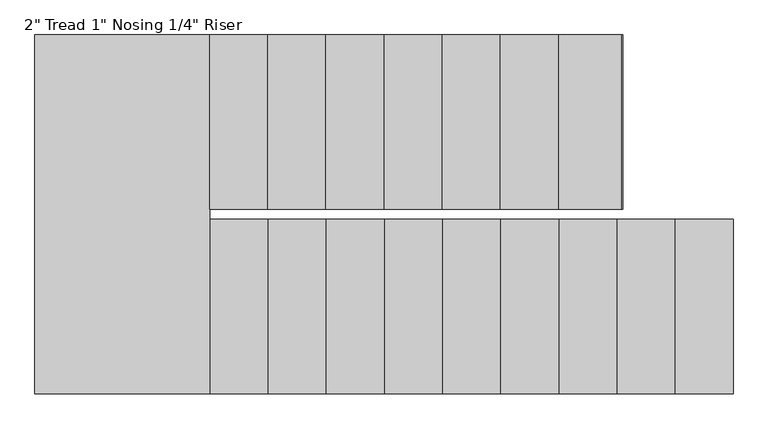
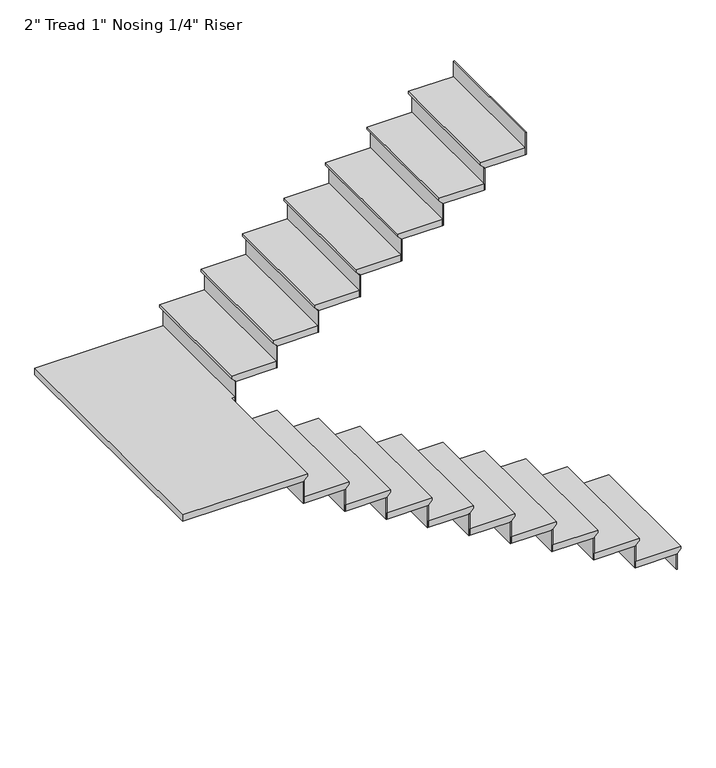
"""IFC4 building model written with IfcOpenShell, lengths in millimetres: stair flight geometry."""

from ifc_helpers import new_model, si_unit, origin, place, context, project, spatial, faceted_brep, source, transform, mapped, element, save


def stair_flight_03b7873a(model_context):
    return source(origin(), model_context, "Body", "Brep", [
        faceted_brep([(-5811.9482439, 2811.8172538, 3503.0833333), (-5811.9482439, 2811.8172538, 3522.1333333), (-5811.9482439, 1897.4172538, 3522.1333333), (-5811.9482439, 1897.4172538, 3503.0833333), (-5837.3482439, 2811.8172538, 3477.6833333), (-5837.3482439, 1897.4172538, 3477.6833333), (-6142.1482439, 2811.8172538, 3522.1333333), (-6142.1482439, 1897.4172538, 3522.1333333), (-5837.3482439, 1897.4172538, 3471.3333333), (-6142.1482439, 1897.4172538, 3471.3333333), (-6142.1482439, 2811.8172538, 3471.3333333), (-5837.3482439, 2811.8172538, 3471.3333333)], [[[0, 1, 2, 3]], [[4, 0, 3, 5]], [[2, 1, 6, 7]], [[8, 9, 10, 11]], [[2, 7, 9, 8, 5, 3]], [[8, 11, 4, 5]], [[6, 1, 0, 4, 11, 10]], [[7, 6, 10, 9]]]),
        faceted_brep([(-5837.3482439, 2811.8172538, 3471.3333333), (-5837.3482439, 2811.8172538, 3352.8), (-5843.6982439, 2811.8172538, 3352.8), (-5843.6982439, 2811.8172538, 3471.3333333), (-5837.3482439, 1897.4172538, 3471.3333333), (-5843.6982439, 1897.4172538, 3471.3333333), (-5843.6982439, 1897.4172538, 3352.8), (-5837.3482439, 1897.4172538, 3352.8)], [[[0, 1, 2, 3]], [[4, 5, 6, 7]], [[1, 0, 4, 7]], [[2, 1, 7, 6]], [[3, 2, 6, 5]], [[0, 3, 5, 4]]]),
        faceted_brep([(-6142.1482439, 2811.8172538, 3640.6666667), (-6142.1482439, 2811.8172538, 3471.3333333), (-6148.4982439, 2811.8172538, 3471.3333333), (-6148.4982439, 2811.8172538, 3640.6666667), (-6142.1482439, 1897.4172538, 3640.6666667), (-6148.4982439, 1897.4172538, 3640.6666667), (-6148.4982439, 1897.4172538, 3471.3333333), (-6142.1482439, 1897.4172538, 3471.3333333)], [[[0, 1, 2, 3]], [[4, 5, 6, 7]], [[1, 0, 4, 7]], [[2, 1, 7, 6]], [[3, 2, 6, 5]], [[0, 3, 5, 4]]]),
        faceted_brep([(-6116.7482439, 1897.4172538, 3691.4666667), (-6116.7482439, 2811.8172538, 3691.4666667), (-6446.9482439, 2811.8172538, 3691.4666667), (-6446.9482439, 1897.4172538, 3691.4666667), (-6142.1482439, 1897.4172538, 3640.6666667), (-6446.9482439, 1897.4172538, 3640.6666667), (-6446.9482439, 2811.8172538, 3640.6666667), (-6142.1482439, 2811.8172538, 3640.6666667), (-6142.1482439, 1897.4172538, 3647.0166667), (-6116.7482439, 1897.4172538, 3672.4166667), (-6142.1482439, 2811.8172538, 3647.0166667), (-6116.7482439, 2811.8172538, 3672.4166667)], [[[0, 1, 2, 3]], [[4, 5, 6, 7]], [[0, 3, 5, 4, 8, 9]], [[4, 7, 10, 8]], [[2, 1, 11, 10, 7, 6]], [[3, 2, 6, 5]], [[11, 1, 0, 9]], [[10, 11, 9, 8]]]),
        faceted_brep([(-6446.9482439, 2811.8172538, 3810.0), (-6446.9482439, 2811.8172538, 3640.6666667), (-6453.2982439, 2811.8172538, 3640.6666667), (-6453.2982439, 2811.8172538, 3810.0), (-6446.9482439, 1897.4172538, 3810.0), (-6453.2982439, 1897.4172538, 3810.0), (-6453.2982439, 1897.4172538, 3640.6666667), (-6446.9482439, 1897.4172538, 3640.6666667)], [[[0, 1, 2, 3]], [[4, 5, 6, 7]], [[1, 0, 4, 7]], [[2, 1, 7, 6]], [[3, 2, 6, 5]], [[0, 3, 5, 4]]]),
        faceted_brep([(-6421.5482439, 1897.4172538, 3860.8), (-6421.5482439, 2811.8172538, 3860.8), (-6751.7482439, 2811.8172538, 3860.8), (-6751.7482439, 1897.4172538, 3860.8), (-6446.9482439, 1897.4172538, 3810.0), (-6751.7482439, 1897.4172538, 3810.0), (-6751.7482439, 2811.8172538, 3810.0), (-6446.9482439, 2811.8172538, 3810.0), (-6446.9482439, 1897.4172538, 3816.35), (-6421.5482439, 1897.4172538, 3841.75), (-6446.9482439, 2811.8172538, 3816.35), (-6421.5482439, 2811.8172538, 3841.75)], [[[0, 1, 2, 3]], [[4, 5, 6, 7]], [[0, 3, 5, 4, 8, 9]], [[4, 7, 10, 8]], [[2, 1, 11, 10, 7, 6]], [[3, 2, 6, 5]], [[11, 1, 0, 9]], [[10, 11, 9, 8]]]),
        faceted_brep([(-6751.7482439, 2811.8172538, 3979.3333333), (-6751.7482439, 2811.8172538, 3810.0), (-6758.0982439, 2811.8172538, 3810.0), (-6758.0982439, 2811.8172538, 3979.3333333), (-6751.7482439, 1897.4172538, 3979.3333333), (-6758.0982439, 1897.4172538, 3979.3333333), (-6758.0982439, 1897.4172538, 3810.0), (-6751.7482439, 1897.4172538, 3810.0)], [[[0, 1, 2, 3]], [[4, 5, 6, 7]], [[1, 0, 4, 7]], [[2, 1, 7, 6]], [[3, 2, 6, 5]], [[0, 3, 5, 4]]]),
        faceted_brep([(-6726.3482439, 1897.4172538, 4030.1333333), (-6726.3482439, 2811.8172538, 4030.1333333), (-7056.5482439, 2811.8172538, 4030.1333333), (-7056.5482439, 1897.4172538, 4030.1333333), (-6751.7482439, 1897.4172538, 3979.3333333), (-7056.5482439, 1897.4172538, 3979.3333333), (-7056.5482439, 2811.8172538, 3979.3333333), (-6751.7482439, 2811.8172538, 3979.3333333), (-6751.7482439, 1897.4172538, 3985.6833333), (-6726.3482439, 1897.4172538, 4011.0833333), (-6751.7482439, 2811.8172538, 3985.6833333), (-6726.3482439, 2811.8172538, 4011.0833333)], [[[0, 1, 2, 3]], [[4, 5, 6, 7]], [[0, 3, 5, 4, 8, 9]], [[4, 7, 10, 8]], [[2, 1, 11, 10, 7, 6]], [[3, 2, 6, 5]], [[11, 1, 0, 9]], [[10, 11, 9, 8]]]),
        faceted_brep([(-7056.5482439, 2811.8172538, 4148.6666667), (-7056.5482439, 2811.8172538, 3979.3333333), (-7062.8982439, 2811.8172538, 3979.3333333), (-7062.8982439, 2811.8172538, 4148.6666667), (-7056.5482439, 1897.4172538, 4148.6666667), (-7062.8982439, 1897.4172538, 4148.6666667), (-7062.8982439, 1897.4172538, 3979.3333333), (-7056.5482439, 1897.4172538, 3979.3333333)], [[[0, 1, 2, 3]], [[4, 5, 6, 7]], [[1, 0, 4, 7]], [[2, 1, 7, 6]], [[3, 2, 6, 5]], [[0, 3, 5, 4]]]),
        faceted_brep([(-7031.1482439, 1897.4172538, 4199.4666667), (-7031.1482439, 2811.8172538, 4199.4666667), (-7361.3482439, 2811.8172538, 4199.4666667), (-7361.3482439, 1897.4172538, 4199.4666667), (-7056.5482439, 1897.4172538, 4148.6666667), (-7361.3482439, 1897.4172538, 4148.6666667), (-7361.3482439, 2811.8172538, 4148.6666667), (-7056.5482439, 2811.8172538, 4148.6666667), (-7056.5482439, 1897.4172538, 4155.0166667), (-7031.1482439, 1897.4172538, 4180.4166667), (-7056.5482439, 2811.8172538, 4155.0166667), (-7031.1482439, 2811.8172538, 4180.4166667)], [[[0, 1, 2, 3]], [[4, 5, 6, 7]], [[0, 3, 5, 4, 8, 9]], [[4, 7, 10, 8]], [[2, 1, 11, 10, 7, 6]], [[3, 2, 6, 5]], [[11, 1, 0, 9]], [[10, 11, 9, 8]]]),
        faceted_brep([(-7361.3482439, 2811.8172538, 4318.0), (-7361.3482439, 2811.8172538, 4148.6666667), (-7367.6982439, 2811.8172538, 4148.6666667), (-7367.6982439, 2811.8172538, 4318.0), (-7361.3482439, 1897.4172538, 4318.0), (-7367.6982439, 1897.4172538, 4318.0), (-7367.6982439, 1897.4172538, 4148.6666667), (-7361.3482439, 1897.4172538, 4148.6666667)], [[[0, 1, 2, 3]], [[4, 5, 6, 7]], [[1, 0, 4, 7]], [[2, 1, 7, 6]], [[3, 2, 6, 5]], [[0, 3, 5, 4]]]),
        faceted_brep([(-7335.9482439, 1897.4172538, 4368.8), (-7335.9482439, 2811.8172538, 4368.8), (-7666.1482439, 2811.8172538, 4368.8), (-7666.1482439, 1897.4172538, 4368.8), (-7361.3482439, 1897.4172538, 4318.0), (-7666.1482439, 1897.4172538, 4318.0), (-7666.1482439, 2811.8172538, 4318.0), (-7361.3482439, 2811.8172538, 4318.0), (-7361.3482439, 1897.4172538, 4324.35), (-7335.9482439, 1897.4172538, 4349.75), (-7361.3482439, 2811.8172538, 4324.35), (-7335.9482439, 2811.8172538, 4349.75)], [[[0, 1, 2, 3]], [[4, 5, 6, 7]], [[0, 3, 5, 4, 8, 9]], [[4, 7, 10, 8]], [[2, 1, 11, 10, 7, 6]], [[3, 2, 6, 5]], [[11, 1, 0, 9]], [[10, 11, 9, 8]]]),
        faceted_brep([(-7666.1482439, 2811.8172538, 4487.3333333), (-7666.1482439, 2811.8172538, 4318.0), (-7672.4982439, 2811.8172538, 4318.0), (-7672.4982439, 2811.8172538, 4487.3333333), (-7666.1482439, 1897.4172538, 4487.3333333), (-7672.4982439, 1897.4172538, 4487.3333333), (-7672.4982439, 1897.4172538, 4318.0), (-7666.1482439, 1897.4172538, 4318.0)], [[[0, 1, 2, 3]], [[4, 5, 6, 7]], [[1, 0, 4, 7]], [[2, 1, 7, 6]], [[3, 2, 6, 5]], [[0, 3, 5, 4]]]),
        faceted_brep([(-7640.7482439, 1897.4172538, 4538.1333333), (-7640.7482439, 2811.8172538, 4538.1333333), (-7970.9482439, 2811.8172538, 4538.1333333), (-7970.9482439, 1897.4172538, 4538.1333333), (-7666.1482439, 1897.4172538, 4487.3333333), (-7970.9482439, 1897.4172538, 4487.3333333), (-7970.9482439, 2811.8172538, 4487.3333333), (-7666.1482439, 2811.8172538, 4487.3333333), (-7666.1482439, 1897.4172538, 4493.6833333), (-7640.7482439, 1897.4172538, 4519.0833333), (-7666.1482439, 2811.8172538, 4493.6833333), (-7640.7482439, 2811.8172538, 4519.0833333)], [[[0, 1, 2, 3]], [[4, 5, 6, 7]], [[0, 3, 5, 4, 8, 9]], [[4, 7, 10, 8]], [[2, 1, 11, 10, 7, 6]], [[3, 2, 6, 5]], [[11, 1, 0, 9]], [[10, 11, 9, 8]]]),
        faceted_brep([(-7970.9482439, 2811.8172538, 4656.6666667), (-7970.9482439, 2811.8172538, 4487.3333333), (-7977.2982439, 2811.8172538, 4487.3333333), (-7977.2982439, 2811.8172538, 4656.6666667), (-7970.9482439, 1897.4172538, 4656.6666667), (-7977.2982439, 1897.4172538, 4656.6666667), (-7977.2982439, 1897.4172538, 4487.3333333), (-7970.9482439, 1897.4172538, 4487.3333333)], [[[0, 1, 2, 3]], [[4, 5, 6, 7]], [[1, 0, 4, 7]], [[2, 1, 7, 6]], [[3, 2, 6, 5]], [[0, 3, 5, 4]]]),
        faceted_brep([(-7945.5482439, 1897.4172538, 4707.4666667), (-7945.5482439, 2811.8172538, 4707.4666667), (-8275.7482439, 2811.8172538, 4707.4666667), (-8275.7482439, 1897.4172538, 4707.4666667), (-7970.9482439, 1897.4172538, 4656.6666667), (-8275.7482439, 1897.4172538, 4656.6666667), (-8275.7482439, 2811.8172538, 4656.6666667), (-7970.9482439, 2811.8172538, 4656.6666667), (-7970.9482439, 1897.4172538, 4663.0166667), (-7945.5482439, 1897.4172538, 4688.4166667), (-7970.9482439, 2811.8172538, 4663.0166667), (-7945.5482439, 2811.8172538, 4688.4166667)], [[[0, 1, 2, 3]], [[4, 5, 6, 7]], [[0, 3, 5, 4, 8, 9]], [[4, 7, 10, 8]], [[2, 1, 11, 10, 7, 6]], [[3, 2, 6, 5]], [[11, 1, 0, 9]], [[10, 11, 9, 8]]]),
        faceted_brep([(-8275.7482439, 2811.8172538, 4826.0), (-8275.7482439, 2811.8172538, 4656.6666667), (-8282.0982439, 2811.8172538, 4656.6666667), (-8282.0982439, 2811.8172538, 4826.0), (-8275.7482439, 1897.4172538, 4826.0), (-8282.0982439, 1897.4172538, 4826.0), (-8282.0982439, 1897.4172538, 4656.6666667), (-8275.7482439, 1897.4172538, 4656.6666667)], [[[0, 1, 2, 3]], [[4, 5, 6, 7]], [[1, 0, 4, 7]], [[2, 1, 7, 6]], [[3, 2, 6, 5]], [[0, 3, 5, 4]]]),
        faceted_brep([(-8250.3482439, 1897.4172538, 4876.8), (-8250.3482439, 2811.8172538, 4876.8), (-8580.5482439, 2811.8172538, 4876.8), (-8580.5482439, 1897.4172538, 4876.8), (-8275.7482439, 1897.4172538, 4826.0), (-8580.5482439, 1897.4172538, 4826.0), (-8580.5482439, 2811.8172538, 4826.0), (-8275.7482439, 2811.8172538, 4826.0), (-8275.7482439, 1897.4172538, 4832.35), (-8250.3482439, 1897.4172538, 4857.75), (-8275.7482439, 2811.8172538, 4832.35), (-8250.3482439, 2811.8172538, 4857.75)], [[[0, 1, 2, 3]], [[4, 5, 6, 7]], [[0, 3, 5, 4, 8, 9]], [[4, 7, 10, 8]], [[2, 1, 11, 10, 7, 6]], [[3, 2, 6, 5]], [[11, 1, 0, 9]], [[10, 11, 9, 8]]]),
        faceted_brep([(-8580.5482439, 2811.8172538, 4995.3333333), (-8580.5482439, 2811.8172538, 4826.0), (-8586.8982439, 2811.8172538, 4826.0), (-8586.8982439, 2811.8172538, 4995.3333333), (-8580.5482439, 1897.4172538, 4995.3333333), (-8586.8982439, 1897.4172538, 4995.3333333), (-8586.8982439, 1897.4172538, 4826.0), (-8580.5482439, 1897.4172538, 4826.0)], [[[0, 1, 2, 3]], [[4, 5, 6, 7]], [[1, 0, 4, 7]], [[2, 1, 7, 6]], [[3, 2, 6, 5]], [[0, 3, 5, 4]]]),
        faceted_brep([(-8529.7482439, 3777.0172538, 5046.1333333), (-9471.1357439, 3777.0172538, 5046.1333333), (-9471.1357439, 1897.4172538, 5046.1333333), (-8555.1482439, 1897.4172538, 5046.1333333), (-8555.1482439, 2862.6172538, 5046.1333333), (-8529.7482439, 2862.6172538, 5046.1333333), (-9471.1357439, 3777.0172538, 4995.3333333), (-8529.7482439, 3777.0172538, 4995.3333333), (-8529.7482439, 2862.6172538, 4995.3333333), (-8555.1482439, 2862.6172538, 4995.3333333), (-8555.1482439, 2811.8172538, 4995.3333333), (-8580.5482439, 2811.8172538, 4995.3333333), (-8580.5482439, 1897.4172538, 4995.3333333), (-9471.1357439, 1897.4172538, 4995.3333333), (-8580.5482439, 1897.4172538, 5001.6833333), (-8555.1482439, 1897.4172538, 5027.0833333), (-8580.5482439, 2811.8172538, 5001.6833333), (-8555.1482439, 2811.8172538, 5027.0833333)], [[[0, 1, 2, 3, 4, 5]], [[6, 7, 8, 9, 10, 11, 12, 13]], [[1, 0, 7, 6]], [[2, 1, 6, 13]], [[3, 2, 13, 12, 14, 15]], [[12, 11, 16, 14]], [[11, 10, 17, 16]], [[4, 3, 15, 17, 10, 9]], [[5, 4, 9, 8]], [[0, 5, 8, 7]], [[15, 14, 16, 17]]]),
        faceted_brep([(-8529.7482439, 2862.6172538, 5164.6666667), (-8529.7482439, 2862.6172538, 4995.3333333), (-8523.3982439, 2862.6172538, 4995.3333333), (-8523.3982439, 2862.6172538, 5164.6666667), (-8529.7482439, 3777.0172538, 5164.6666667), (-8523.3982439, 3777.0172538, 5164.6666667), (-8523.3982439, 3777.0172538, 4995.3333333), (-8529.7482439, 3777.0172538, 4995.3333333)], [[[0, 1, 2, 3]], [[4, 5, 6, 7]], [[1, 0, 4, 7]], [[2, 1, 7, 6]], [[3, 2, 6, 5]], [[0, 3, 5, 4]]]),
        faceted_brep([(-8555.1482439, 3777.0172538, 5215.4666667), (-8555.1482439, 2862.6172538, 5215.4666667), (-8224.9482439, 2862.6172538, 5215.4666667), (-8224.9482439, 3777.0172538, 5215.4666667), (-8529.7482439, 3777.0172538, 5164.6666667), (-8224.9482439, 3777.0172538, 5164.6666667), (-8224.9482439, 2862.6172538, 5164.6666667), (-8529.7482439, 2862.6172538, 5164.6666667), (-8529.7482439, 3777.0172538, 5171.0166667), (-8555.1482439, 3777.0172538, 5196.4166667), (-8529.7482439, 2862.6172538, 5171.0166667), (-8555.1482439, 2862.6172538, 5196.4166667)], [[[0, 1, 2, 3]], [[4, 5, 6, 7]], [[0, 3, 5, 4, 8, 9]], [[4, 7, 10, 8]], [[2, 1, 11, 10, 7, 6]], [[3, 2, 6, 5]], [[11, 1, 0, 9]], [[10, 11, 9, 8]]]),
        faceted_brep([(-8224.9482439, 2862.6172538, 5334.0), (-8224.9482439, 2862.6172538, 5164.6666667), (-8218.5982439, 2862.6172538, 5164.6666667), (-8218.5982439, 2862.6172538, 5334.0), (-8224.9482439, 3777.0172538, 5334.0), (-8218.5982439, 3777.0172538, 5334.0), (-8218.5982439, 3777.0172538, 5164.6666667), (-8224.9482439, 3777.0172538, 5164.6666667)], [[[0, 1, 2, 3]], [[4, 5, 6, 7]], [[1, 0, 4, 7]], [[2, 1, 7, 6]], [[3, 2, 6, 5]], [[0, 3, 5, 4]]]),
        faceted_brep([(-8250.3482439, 3777.0172538, 5384.8), (-8250.3482439, 2862.6172538, 5384.8), (-7920.1482439, 2862.6172538, 5384.8), (-7920.1482439, 3777.0172538, 5384.8), (-8224.9482439, 3777.0172538, 5334.0), (-7920.1482439, 3777.0172538, 5334.0), (-7920.1482439, 2862.6172538, 5334.0), (-8224.9482439, 2862.6172538, 5334.0), (-8224.9482439, 3777.0172538, 5340.35), (-8250.3482439, 3777.0172538, 5365.75), (-8224.9482439, 2862.6172538, 5340.35), (-8250.3482439, 2862.6172538, 5365.75)], [[[0, 1, 2, 3]], [[4, 5, 6, 7]], [[0, 3, 5, 4, 8, 9]], [[4, 7, 10, 8]], [[2, 1, 11, 10, 7, 6]], [[3, 2, 6, 5]], [[11, 1, 0, 9]], [[10, 11, 9, 8]]]),
        faceted_brep([(-7920.1482439, 2862.6172538, 5503.3333333), (-7920.1482439, 2862.6172538, 5334.0), (-7913.7982439, 2862.6172538, 5334.0), (-7913.7982439, 2862.6172538, 5503.3333333), (-7920.1482439, 3777.0172538, 5503.3333333), (-7913.7982439, 3777.0172538, 5503.3333333), (-7913.7982439, 3777.0172538, 5334.0), (-7920.1482439, 3777.0172538, 5334.0)], [[[0, 1, 2, 3]], [[4, 5, 6, 7]], [[1, 0, 4, 7]], [[2, 1, 7, 6]], [[3, 2, 6, 5]], [[0, 3, 5, 4]]]),
        faceted_brep([(-7945.5482439, 3777.0172538, 5554.1333333), (-7945.5482439, 2862.6172538, 5554.1333333), (-7615.3482439, 2862.6172538, 5554.1333333), (-7615.3482439, 3777.0172538, 5554.1333333), (-7920.1482439, 3777.0172538, 5503.3333333), (-7615.3482439, 3777.0172538, 5503.3333333), (-7615.3482439, 2862.6172538, 5503.3333333), (-7920.1482439, 2862.6172538, 5503.3333333), (-7920.1482439, 3777.0172538, 5509.6833333), (-7945.5482439, 3777.0172538, 5535.0833333), (-7920.1482439, 2862.6172538, 5509.6833333), (-7945.5482439, 2862.6172538, 5535.0833333)], [[[0, 1, 2, 3]], [[4, 5, 6, 7]], [[0, 3, 5, 4, 8, 9]], [[4, 7, 10, 8]], [[2, 1, 11, 10, 7, 6]], [[3, 2, 6, 5]], [[11, 1, 0, 9]], [[10, 11, 9, 8]]]),
        faceted_brep([(-7615.3482439, 2862.6172538, 5672.6666667), (-7615.3482439, 2862.6172538, 5503.3333333), (-7608.9982439, 2862.6172538, 5503.3333333), (-7608.9982439, 2862.6172538, 5672.6666667), (-7615.3482439, 3777.0172538, 5672.6666667), (-7608.9982439, 3777.0172538, 5672.6666667), (-7608.9982439, 3777.0172538, 5503.3333333), (-7615.3482439, 3777.0172538, 5503.3333333)], [[[0, 1, 2, 3]], [[4, 5, 6, 7]], [[1, 0, 4, 7]], [[2, 1, 7, 6]], [[3, 2, 6, 5]], [[0, 3, 5, 4]]]),
        faceted_brep([(-7640.7482439, 3777.0172538, 5723.4666667), (-7640.7482439, 2862.6172538, 5723.4666667), (-7310.5482439, 2862.6172538, 5723.4666667), (-7310.5482439, 3777.0172538, 5723.4666667), (-7615.3482439, 3777.0172538, 5672.6666667), (-7310.5482439, 3777.0172538, 5672.6666667), (-7310.5482439, 2862.6172538, 5672.6666667), (-7615.3482439, 2862.6172538, 5672.6666667), (-7615.3482439, 3777.0172538, 5679.0166667), (-7640.7482439, 3777.0172538, 5704.4166667), (-7615.3482439, 2862.6172538, 5679.0166667), (-7640.7482439, 2862.6172538, 5704.4166667)], [[[0, 1, 2, 3]], [[4, 5, 6, 7]], [[0, 3, 5, 4, 8, 9]], [[4, 7, 10, 8]], [[2, 1, 11, 10, 7, 6]], [[3, 2, 6, 5]], [[11, 1, 0, 9]], [[10, 11, 9, 8]]]),
        faceted_brep([(-7310.5482439, 2862.6172538, 5842.0), (-7310.5482439, 2862.6172538, 5672.6666667), (-7304.1982439, 2862.6172538, 5672.6666667), (-7304.1982439, 2862.6172538, 5842.0), (-7310.5482439, 3777.0172538, 5842.0), (-7304.1982439, 3777.0172538, 5842.0), (-7304.1982439, 3777.0172538, 5672.6666667), (-7310.5482439, 3777.0172538, 5672.6666667)], [[[0, 1, 2, 3]], [[4, 5, 6, 7]], [[1, 0, 4, 7]], [[2, 1, 7, 6]], [[3, 2, 6, 5]], [[0, 3, 5, 4]]]),
        faceted_brep([(-7335.9482439, 3777.0172538, 5892.8), (-7335.9482439, 2862.6172538, 5892.8), (-7005.7482439, 2862.6172538, 5892.8), (-7005.7482439, 3777.0172538, 5892.8), (-7310.5482439, 3777.0172538, 5842.0), (-7005.7482439, 3777.0172538, 5842.0), (-7005.7482439, 2862.6172538, 5842.0), (-7310.5482439, 2862.6172538, 5842.0), (-7310.5482439, 3777.0172538, 5848.35), (-7335.9482439, 3777.0172538, 5873.75), (-7310.5482439, 2862.6172538, 5848.35), (-7335.9482439, 2862.6172538, 5873.75)], [[[0, 1, 2, 3]], [[4, 5, 6, 7]], [[0, 3, 5, 4, 8, 9]], [[4, 7, 10, 8]], [[2, 1, 11, 10, 7, 6]], [[3, 2, 6, 5]], [[11, 1, 0, 9]], [[10, 11, 9, 8]]]),
        faceted_brep([(-7005.7482439, 2862.6172538, 6011.3333333), (-7005.7482439, 2862.6172538, 5842.0), (-6999.3982439, 2862.6172538, 5842.0), (-6999.3982439, 2862.6172538, 6011.3333333), (-7005.7482439, 3777.0172538, 6011.3333333), (-6999.3982439, 3777.0172538, 6011.3333333), (-6999.3982439, 3777.0172538, 5842.0), (-7005.7482439, 3777.0172538, 5842.0)], [[[0, 1, 2, 3]], [[4, 5, 6, 7]], [[1, 0, 4, 7]], [[2, 1, 7, 6]], [[3, 2, 6, 5]], [[0, 3, 5, 4]]]),
        faceted_brep([(-7031.1482439, 3777.0172538, 6062.1333333), (-7031.1482439, 2862.6172538, 6062.1333333), (-6700.9482439, 2862.6172538, 6062.1333333), (-6700.9482439, 3777.0172538, 6062.1333333), (-7005.7482439, 3777.0172538, 6011.3333333), (-6700.9482439, 3777.0172538, 6011.3333333), (-6700.9482439, 2862.6172538, 6011.3333333), (-7005.7482439, 2862.6172538, 6011.3333333), (-7005.7482439, 3777.0172538, 6017.6833333), (-7031.1482439, 3777.0172538, 6043.0833333), (-7005.7482439, 2862.6172538, 6017.6833333), (-7031.1482439, 2862.6172538, 6043.0833333)], [[[0, 1, 2, 3]], [[4, 5, 6, 7]], [[0, 3, 5, 4, 8, 9]], [[4, 7, 10, 8]], [[2, 1, 11, 10, 7, 6]], [[3, 2, 6, 5]], [[11, 1, 0, 9]], [[10, 11, 9, 8]]]),
        faceted_brep([(-6700.9482439, 2862.6172538, 6180.6666667), (-6700.9482439, 2862.6172538, 6011.3333333), (-6694.5982439, 2862.6172538, 6011.3333333), (-6694.5982439, 2862.6172538, 6180.6666667), (-6700.9482439, 3777.0172538, 6180.6666667), (-6694.5982439, 3777.0172538, 6180.6666667), (-6694.5982439, 3777.0172538, 6011.3333333), (-6700.9482439, 3777.0172538, 6011.3333333)], [[[0, 1, 2, 3]], [[4, 5, 6, 7]], [[1, 0, 4, 7]], [[2, 1, 7, 6]], [[3, 2, 6, 5]], [[0, 3, 5, 4]]]),
        faceted_brep([(-6396.1482439, 2862.6172538, 6350.0), (-6396.1482439, 2862.6172538, 6180.6666667), (-6389.7982439, 2862.6172538, 6180.6666667), (-6389.7982439, 2862.6172538, 6350.0), (-6396.1482439, 3777.0172538, 6350.0), (-6389.7982439, 3777.0172538, 6350.0), (-6389.7982439, 3777.0172538, 6180.6666667), (-6396.1482439, 3777.0172538, 6180.6666667)], [[[0, 1, 2, 3]], [[4, 5, 6, 7]], [[1, 0, 4, 7]], [[2, 1, 7, 6]], [[3, 2, 6, 5]], [[0, 3, 5, 4]]]),
        faceted_brep([(-6726.3482439, 3777.0172538, 6231.4666667), (-6726.3482439, 2862.6172538, 6231.4666667), (-6396.1482439, 2862.6172538, 6231.4666667), (-6396.1482439, 3777.0172538, 6231.4666667), (-6700.9482439, 3777.0172538, 6180.6666667), (-6396.1482439, 3777.0172538, 6180.6666667), (-6396.1482439, 2862.6172538, 6180.6666667), (-6700.9482439, 2862.6172538, 6180.6666667), (-6700.9482439, 3777.0172538, 6187.0166667), (-6726.3482439, 3777.0172538, 6212.4166667), (-6700.9482439, 2862.6172538, 6187.0166667), (-6726.3482439, 2862.6172538, 6212.4166667)], [[[0, 1, 2, 3]], [[4, 5, 6, 7]], [[0, 3, 5, 4, 8, 9]], [[4, 7, 10, 8]], [[2, 1, 11, 10, 7, 6]], [[3, 2, 6, 5]], [[11, 1, 0, 9]], [[10, 11, 9, 8]]]),
    ])


if __name__ == "__main__":
    model = new_model("IFC4")
    model_context = context("Model", 3, world=origin())
    ifc_project = project(units=[si_unit("LENGTHUNIT", "METRE", prefix="MILLI")], contexts=[model_context])
    site = spatial("IfcSite", under=ifc_project)
    building = spatial("IfcBuilding", under=site)
    placement = place(None, origin())
    stair_flight_shape = stair_flight_03b7873a(model_context)
    element("IfcStairFlight", 1, ObjectType="2\" Tread 1\" Nosing 1/4\" Riser", at=placement, inside=building, context=model_context, shape_type="MappedRepresentation", body=[
        mapped(stair_flight_shape, transform((0.0, 0.0, 0.0), x_axis=(1.0, 0.0, 0.0), y_axis=(0.0, 1.0, 0.0), z_axis=(0.0, 0.0, 1.0))),
    ])
    save(model, "model.ifc")

# Revit data of these elements
# Element 1 (IfcStairFlight, "2\" Tread 1\" Nosing 1/4\" Riser")
#   Materials on its faces: "MARBLE PAINT"
# Materials
#   "MARBLE PAINT": class "Generic", colour RGB 120 120 120, transparency 0, Cost = 0
